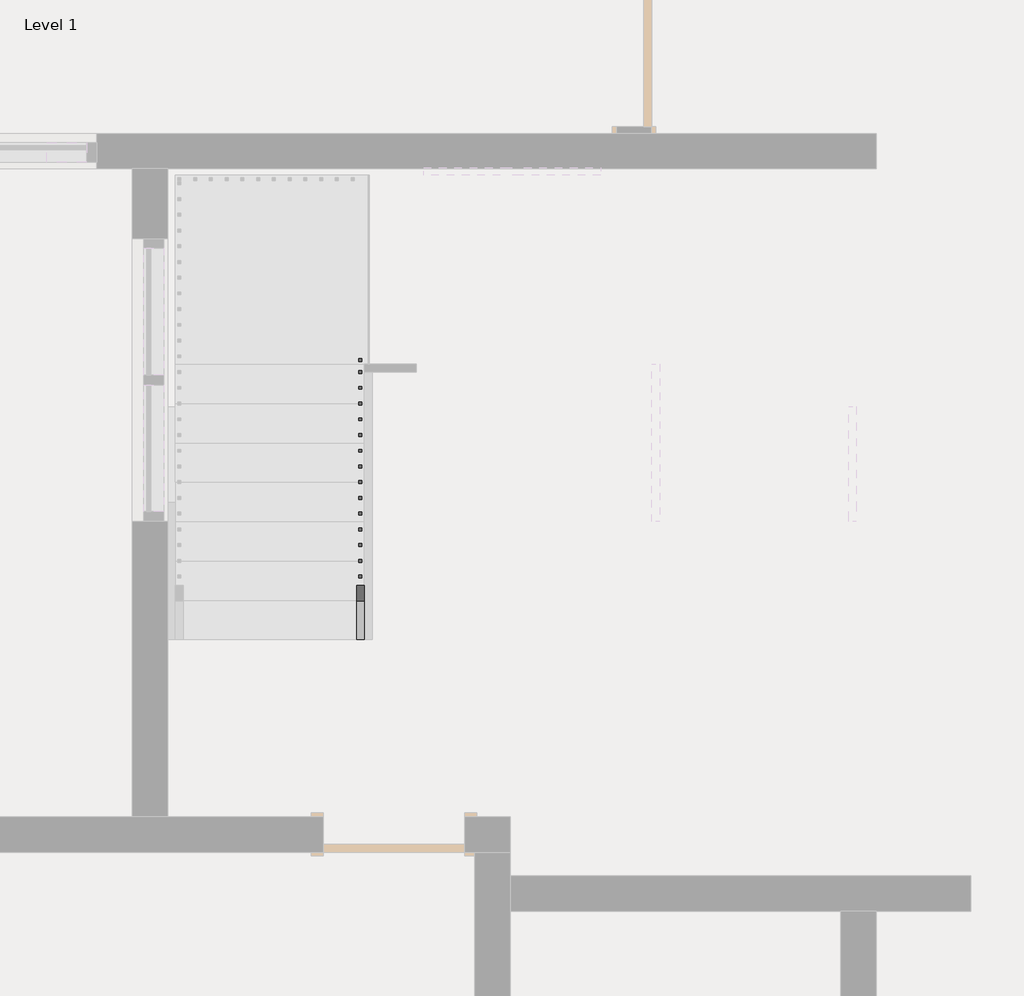
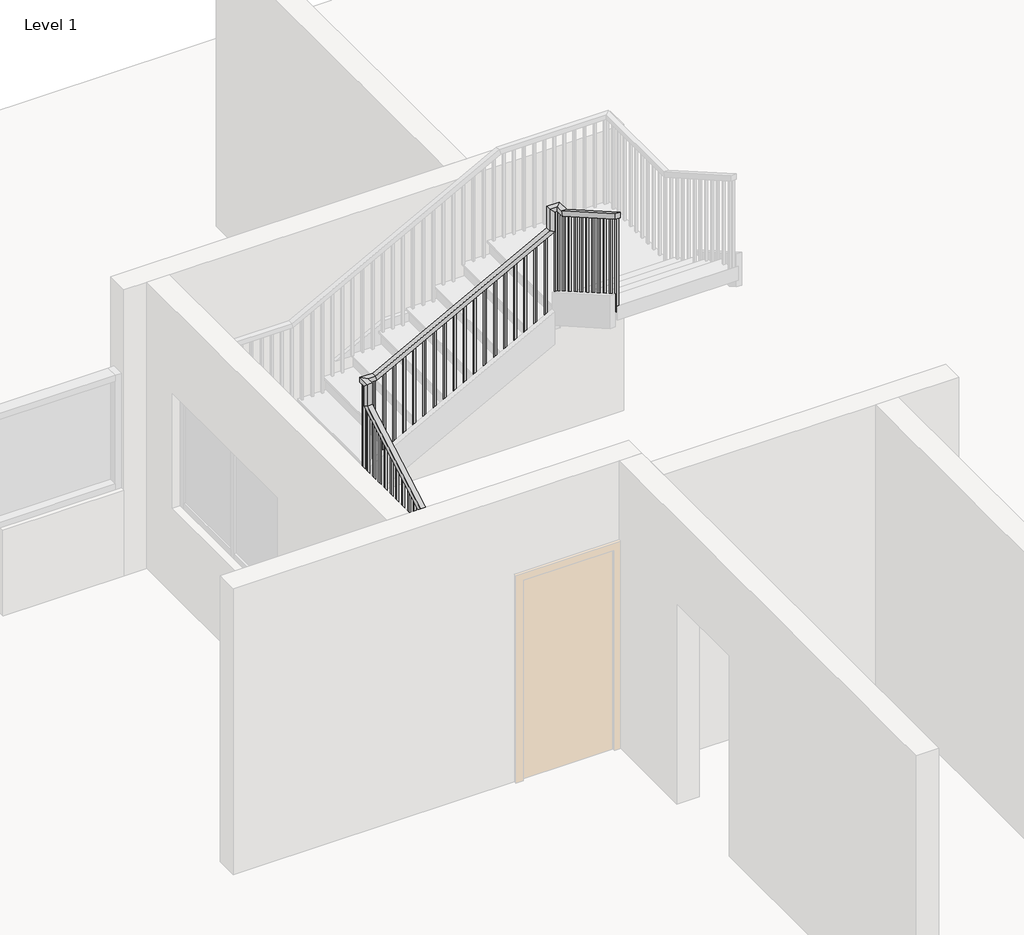
# One storey, part 6 of 9: 1 railing.
"""IFC4 building model written with IfcOpenShell, lengths in millimetres."""

from ifc_helpers import new_model, si_unit, frame, origin, place, context, project, spatial, polyline, outline, extrude, faceted_brep, element, save

model = new_model("IFC4")

# Units and contexts
model_context = context("Model", 3, world=origin())
ifc_project = project(units=[si_unit("LENGTHUNIT", "METRE", prefix="MILLI")], contexts=[model_context])

# Site, building, storey
site = spatial("IfcSite", under=ifc_project)
building = spatial("IfcBuilding", under=site)
storey = spatial("IfcBuildingStorey", under=building, Name="Level 1", Elevation=0.0)

# Railing
placement = place(None, origin())
element("IfcRailing", 1, ObjectType="Handrail - Rectangular", at=placement, inside=storey, context=model_context, shape_type="SolidModel", body=[
    faceted_brep([(-39782.5146233, 12415.3624892, 1059.5428571), (-39782.5146233, 12415.3624892, 1001.0339009), (-39731.7146233, 12415.3624892, 1001.0339009), (-39731.7146233, 12415.3624892, 1059.5428571), (-39782.5146233, 14117.1624892, 2032.0), (-39782.5146233, 14167.9624892, 2002.5196152), (-39731.7146233, 14167.9624892, 2002.5196152), (-39731.7146233, 14117.1624892, 2032.0), (-39782.5146233, 14117.1624892, 2261.3257143), (-39782.5146233, 14167.9624892, 2210.5257143), (-39731.7146233, 14167.9624892, 2210.5257143), (-39731.7146233, 14117.1624892, 2261.3257143), (-39782.5146233, 14244.1624892, 2261.3257143), (-39782.5146233, 14244.1624892, 2210.5257143), (-39731.7146233, 14193.3624892, 2210.5257143), (-39731.7146233, 14193.3624892, 2261.3257143), (-39655.5146233, 14244.1624892, 2261.3257143), (-39642.8146233, 14244.1624892, 2210.5257143), (-39642.8146233, 14193.3624892, 2210.5257143), (-39655.5146233, 14193.3624892, 2261.3257143), (-37902.9146233, 14244.1624892, 3196.0457143), (-37852.1146233, 14244.1624892, 3165.5657143), (-37852.1146233, 14193.3624892, 3165.5657143), (-37902.9146233, 14193.3624892, 3196.0457143), (-37902.9146233, 14244.1624892, 3425.3714286), (-37852.1146233, 14244.1624892, 3374.5714286), (-37852.1146233, 14193.3624892, 3374.5714286), (-37902.9146233, 14193.3624892, 3425.3714286), (-37775.9146233, 14244.1624892, 3425.3714286), (-37775.9146233, 14244.1624892, 3374.5714286), (-37826.7146233, 14193.3624892, 3374.5714286), (-37826.7146233, 14193.3624892, 3425.3714286), (-37775.9146233, 14117.1624892, 3425.3714286), (-37775.9146233, 14103.6718158, 3374.5714286), (-37826.7146233, 14103.6718158, 3374.5714286), (-37826.7146233, 14117.1624892, 3425.3714286), (-37775.9146233, 13177.3624892, 3962.4), (-37826.7146233, 13177.3624892, 3962.4), (-37826.7146233, 13177.3624892, 3903.8910438), (-37775.9146233, 13177.3624892, 3903.8910438)], [[[0, 1, 2, 3]], [[1, 0, 4, 5]], [[2, 1, 5, 6]], [[3, 2, 6, 7]], [[0, 3, 7, 4]], [[5, 4, 8, 9]], [[6, 5, 9, 10]], [[7, 6, 10, 11]], [[4, 7, 11, 8]], [[9, 8, 12, 13]], [[10, 9, 13, 14]], [[11, 10, 14, 15]], [[8, 11, 15, 12]], [[13, 12, 16, 17]], [[14, 13, 17, 18]], [[15, 14, 18, 19]], [[12, 15, 19, 16]], [[17, 16, 20, 21]], [[18, 17, 21, 22]], [[19, 18, 22, 23]], [[16, 19, 23, 20]], [[21, 20, 24, 25]], [[22, 21, 25, 26]], [[23, 22, 26, 27]], [[20, 23, 27, 24]], [[25, 24, 28, 29]], [[26, 25, 29, 30]], [[27, 26, 30, 31]], [[24, 27, 31, 28]], [[29, 28, 32, 33]], [[30, 29, 33, 34]], [[31, 30, 34, 35]], [[28, 31, 35, 32]], [[36, 37, 38, 39]], [[33, 32, 36, 39]], [[34, 33, 39, 38]], [[35, 34, 38, 37]], [[32, 35, 37, 36]]]),
    extrude(outline(polyline([(13193.2374892, 3894.8196152), (13212.2874892, 3883.9339009), (13212.2874892, 2902.8571429), (13193.2374892, 2902.8571429), (13193.2374892, 3894.8196152)])), frame((-37810.8396233, 0.0, 0.0), z_axis=(1.0, 0.0, 0.0), x_axis=(0.0, 1.0, 0.0)), (0.0, 0.0, 1.0), 19.05),
    extrude(outline(polyline([(13294.8374892, 3836.7624723), (13313.8874892, 3825.8767581), (13313.8874892, 2902.8571429), (13294.8374892, 2902.8571429), (13294.8374892, 3836.7624723)])), frame((-37810.8396233, 0.0, 0.0), z_axis=(1.0, 0.0, 0.0), x_axis=(0.0, 1.0, 0.0)), (0.0, 0.0, 1.0), 19.05),
    extrude(outline(polyline([(13396.4374892, 3778.7053295), (13415.4874892, 3767.8196152), (13415.4874892, 2902.8571429), (13396.4374892, 2902.8571429), (13396.4374892, 3778.7053295)])), frame((-37810.8396233, 0.0, 0.0), z_axis=(1.0, 0.0, 0.0), x_axis=(0.0, 1.0, 0.0)), (0.0, 0.0, 1.0), 19.05),
    extrude(outline(polyline([(13498.0374892, 3720.6481866), (13517.0874892, 3709.7624723), (13517.0874892, 2757.7142857), (13498.0374892, 2757.7142857), (13498.0374892, 3720.6481866)])), frame((-37810.8396233, 0.0, 0.0), z_axis=(1.0, 0.0, 0.0), x_axis=(0.0, 1.0, 0.0)), (0.0, 0.0, 1.0), 19.05),
    extrude(outline(polyline([(13599.6374892, 3662.5910438), (13618.6874892, 3651.7053295), (13618.6874892, 2757.7142857), (13599.6374892, 2757.7142857), (13599.6374892, 3662.5910438)])), frame((-37810.8396233, 0.0, 0.0), z_axis=(1.0, 0.0, 0.0), x_axis=(0.0, 1.0, 0.0)), (0.0, 0.0, 1.0), 19.05),
    extrude(outline(polyline([(13701.2374892, 3604.5339009), (13720.2874892, 3593.6481866), (13720.2874892, 2612.5714286), (13701.2374892, 2612.5714286), (13701.2374892, 3604.5339009)])), frame((-37810.8396233, 0.0, 0.0), z_axis=(1.0, 0.0, 0.0), x_axis=(0.0, 1.0, 0.0)), (0.0, 0.0, 1.0), 19.05),
    extrude(outline(polyline([(13802.8374892, 3546.4767581), (13821.8874892, 3535.5910438), (13821.8874892, 2612.5714286), (13802.8374892, 2612.5714286), (13802.8374892, 3546.4767581)])), frame((-37810.8396233, 0.0, 0.0), z_axis=(1.0, 0.0, 0.0), x_axis=(0.0, 1.0, 0.0)), (0.0, 0.0, 1.0), 19.05),
    extrude(outline(polyline([(13904.4374892, 3488.4196152), (13923.4874892, 3477.5339009), (13923.4874892, 2612.5714286), (13904.4374892, 2612.5714286), (13904.4374892, 3488.4196152)])), frame((-37810.8396233, 0.0, 0.0), z_axis=(1.0, 0.0, 0.0), x_axis=(0.0, 1.0, 0.0)), (0.0, 0.0, 1.0), 19.05),
    extrude(outline(polyline([(14006.0374892, 3430.3624723), (14025.0874892, 3419.4767581), (14025.0874892, 2467.4285714), (14006.0374892, 2467.4285714), (14006.0374892, 3430.3624723)])), frame((-37810.8396233, 0.0, 0.0), z_axis=(1.0, 0.0, 0.0), x_axis=(0.0, 1.0, 0.0)), (0.0, 0.0, 1.0), 19.05),
    extrude(outline(polyline([(14107.6374892, 3372.3053295), (14126.6874892, 3361.4196152), (14126.6874892, 2467.4285714), (14107.6374892, 2467.4285714), (14107.6374892, 3372.3053295)])), frame((-37810.8396233, 0.0, 0.0), z_axis=(1.0, 0.0, 0.0), x_axis=(0.0, 1.0, 0.0)), (0.0, 0.0, 1.0), 19.05),
    extrude(outline(polyline([(-37836.2396233, 14209.2374892), (-37836.2396233, 14228.2874892), (-37817.1896233, 14228.2874892), (-37817.1896233, 14209.2374892), (-37836.2396233, 14209.2374892)])), frame((0.0, 0.0, 2322.2857143), z_axis=(0.0, 0.0, 1.0), x_axis=(1.0, 0.0, 0.0)), (0.0, 0.0, 1.0), 1052.2857143),
    extrude(outline(polyline([(3130.0057143, -37918.7896233), (3119.8457143, -37937.8396233), (2177.1428571, -37937.8396233), (2177.1428571, -37918.7896233), (3130.0057143, -37918.7896233)])), frame((0.0, 14209.2374892, 0.0), z_axis=(0.0, 1.0, 0.0), x_axis=(0.0, 0.0, 1.0)), (0.0, 0.0, 1.0), 19.05),
    extrude(outline(polyline([(3075.8190476, -38020.3896233), (3065.6590476, -38039.4396233), (2177.1428571, -38039.4396233), (2177.1428571, -38020.3896233), (3075.8190476, -38020.3896233)])), frame((0.0, 14209.2374892, 0.0), z_axis=(0.0, 1.0, 0.0), x_axis=(0.0, 0.0, 1.0)), (0.0, 0.0, 1.0), 19.05),
    extrude(outline(polyline([(3021.632381, -38121.9896233), (3011.472381, -38141.0396233), (2032.0, -38141.0396233), (2032.0, -38121.9896233), (3021.632381, -38121.9896233)])), frame((0.0, 14209.2374892, 0.0), z_axis=(0.0, 1.0, 0.0), x_axis=(0.0, 0.0, 1.0)), (0.0, 0.0, 1.0), 19.05),
    extrude(outline(polyline([(2967.4457143, -38223.5896233), (2957.2857143, -38242.6396233), (2032.0, -38242.6396233), (2032.0, -38223.5896233), (2967.4457143, -38223.5896233)])), frame((0.0, 14209.2374892, 0.0), z_axis=(0.0, 1.0, 0.0), x_axis=(0.0, 0.0, 1.0)), (0.0, 0.0, 1.0), 19.05),
    extrude(outline(polyline([(2913.2590476, -38325.1896233), (2903.0990476, -38344.2396233), (2032.0, -38344.2396233), (2032.0, -38325.1896233), (2913.2590476, -38325.1896233)])), frame((0.0, 14209.2374892, 0.0), z_axis=(0.0, 1.0, 0.0), x_axis=(0.0, 0.0, 1.0)), (0.0, 0.0, 1.0), 19.05),
    extrude(outline(polyline([(2859.072381, -38426.7896233), (2848.912381, -38445.8396233), (1886.8571429, -38445.8396233), (1886.8571429, -38426.7896233), (2859.072381, -38426.7896233)])), frame((0.0, 14209.2374892, 0.0), z_axis=(0.0, 1.0, 0.0), x_axis=(0.0, 0.0, 1.0)), (0.0, 0.0, 1.0), 19.05),
    extrude(outline(polyline([(2804.8857143, -38528.3896233), (2794.7257143, -38547.4396233), (1886.8571429, -38547.4396233), (1886.8571429, -38528.3896233), (2804.8857143, -38528.3896233)])), frame((0.0, 14209.2374892, 0.0), z_axis=(0.0, 1.0, 0.0), x_axis=(0.0, 0.0, 1.0)), (0.0, 0.0, 1.0), 19.05),
    extrude(outline(polyline([(2750.6990476, -38629.9896233), (2740.5390476, -38649.0396233), (1886.8571429, -38649.0396233), (1886.8571429, -38629.9896233), (2750.6990476, -38629.9896233)])), frame((0.0, 14209.2374892, 0.0), z_axis=(0.0, 1.0, 0.0), x_axis=(0.0, 0.0, 1.0)), (0.0, 0.0, 1.0), 19.05),
    extrude(outline(polyline([(2696.512381, -38731.5896233), (2686.352381, -38750.6396233), (1741.7142857, -38750.6396233), (1741.7142857, -38731.5896233), (2696.512381, -38731.5896233)])), frame((0.0, 14209.2374892, 0.0), z_axis=(0.0, 1.0, 0.0), x_axis=(0.0, 0.0, 1.0)), (0.0, 0.0, 1.0), 19.05),
    extrude(outline(polyline([(2642.3257143, -38833.1896233), (2632.1657143, -38852.2396233), (1741.7142857, -38852.2396233), (1741.7142857, -38833.1896233), (2642.3257143, -38833.1896233)])), frame((0.0, 14209.2374892, 0.0), z_axis=(0.0, 1.0, 0.0), x_axis=(0.0, 0.0, 1.0)), (0.0, 0.0, 1.0), 19.05),
    extrude(outline(polyline([(2588.1390476, -38934.7896233), (2577.9790476, -38953.8396233), (1596.5714286, -38953.8396233), (1596.5714286, -38934.7896233), (2588.1390476, -38934.7896233)])), frame((0.0, 14209.2374892, 0.0), z_axis=(0.0, 1.0, 0.0), x_axis=(0.0, 0.0, 1.0)), (0.0, 0.0, 1.0), 19.05),
    extrude(outline(polyline([(2533.952381, -39036.3896233), (2523.792381, -39055.4396233), (1596.5714286, -39055.4396233), (1596.5714286, -39036.3896233), (2533.952381, -39036.3896233)])), frame((0.0, 14209.2374892, 0.0), z_axis=(0.0, 1.0, 0.0), x_axis=(0.0, 0.0, 1.0)), (0.0, 0.0, 1.0), 19.05),
    extrude(outline(polyline([(2479.7657143, -39137.9896233), (2469.6057143, -39157.0396233), (1596.5714286, -39157.0396233), (1596.5714286, -39137.9896233), (2479.7657143, -39137.9896233)])), frame((0.0, 14209.2374892, 0.0), z_axis=(0.0, 1.0, 0.0), x_axis=(0.0, 0.0, 1.0)), (0.0, 0.0, 1.0), 19.05),
    extrude(outline(polyline([(2425.5790476, -39239.5896233), (2415.4190476, -39258.6396233), (1451.4285714, -39258.6396233), (1451.4285714, -39239.5896233), (2425.5790476, -39239.5896233)])), frame((0.0, 14209.2374892, 0.0), z_axis=(0.0, 1.0, 0.0), x_axis=(0.0, 0.0, 1.0)), (0.0, 0.0, 1.0), 19.05),
    extrude(outline(polyline([(2371.392381, -39341.1896233), (2361.232381, -39360.2396233), (1451.4285714, -39360.2396233), (1451.4285714, -39341.1896233), (2371.392381, -39341.1896233)])), frame((0.0, 14209.2374892, 0.0), z_axis=(0.0, 1.0, 0.0), x_axis=(0.0, 0.0, 1.0)), (0.0, 0.0, 1.0), 19.05),
    extrude(outline(polyline([(2317.2057143, -39442.7896233), (2307.0457143, -39461.8396233), (1451.4285714, -39461.8396233), (1451.4285714, -39442.7896233), (2317.2057143, -39442.7896233)])), frame((0.0, 14209.2374892, 0.0), z_axis=(0.0, 1.0, 0.0), x_axis=(0.0, 0.0, 1.0)), (0.0, 0.0, 1.0), 19.05),
    extrude(outline(polyline([(2263.0190476, -39544.3896233), (2252.8590476, -39563.4396233), (1306.2857143, -39563.4396233), (1306.2857143, -39544.3896233), (2263.0190476, -39544.3896233)])), frame((0.0, 14209.2374892, 0.0), z_axis=(0.0, 1.0, 0.0), x_axis=(0.0, 0.0, 1.0)), (0.0, 0.0, 1.0), 19.05),
    extrude(outline(polyline([(2208.832381, -39645.9896233), (2198.672381, -39665.0396233), (1306.2857143, -39665.0396233), (1306.2857143, -39645.9896233), (2208.832381, -39645.9896233)])), frame((0.0, 14209.2374892, 0.0), z_axis=(0.0, 1.0, 0.0), x_axis=(0.0, 0.0, 1.0)), (0.0, 0.0, 1.0), 19.05),
    extrude(outline(polyline([(-39747.5896233, 14133.0374892), (-39766.6396233, 14133.0374892), (-39766.6396233, 14152.0874892), (-39747.5896233, 14152.0874892), (-39747.5896233, 14133.0374892)])), frame((0.0, 0.0, 1016.0), z_axis=(0.0, 0.0, 1.0), x_axis=(1.0, 0.0, 0.0)), (0.0, 0.0, 1.0), 1194.5257143),
    extrude(outline(polyline([(14031.4374892, 1924.5053295), (14050.4874892, 1935.3910438), (14050.4874892, 1016.0), (14031.4374892, 1016.0), (14031.4374892, 1924.5053295)])), frame((-39766.6396233, 0.0, 0.0), z_axis=(1.0, 0.0, 0.0), x_axis=(0.0, 1.0, 0.0)), (0.0, 0.0, 1.0), 19.05),
    extrude(outline(polyline([(13929.8374892, 1866.4481866), (13948.8874892, 1877.3339009), (13948.8874892, 1016.0), (13929.8374892, 1016.0), (13929.8374892, 1866.4481866)])), frame((-39766.6396233, 0.0, 0.0), z_axis=(1.0, 0.0, 0.0), x_axis=(0.0, 1.0, 0.0)), (0.0, 0.0, 1.0), 19.05),
    extrude(outline(polyline([(13828.2374892, 1808.3910438), (13847.2874892, 1819.2767581), (13847.2874892, 870.8571429), (13828.2374892, 870.8571429), (13828.2374892, 1808.3910438)])), frame((-39766.6396233, 0.0, 0.0), z_axis=(1.0, 0.0, 0.0), x_axis=(0.0, 1.0, 0.0)), (0.0, 0.0, 1.0), 19.05),
    extrude(outline(polyline([(13726.6374892, 1750.3339009), (13745.6874892, 1761.2196152), (13745.6874892, 870.8571429), (13726.6374892, 870.8571429), (13726.6374892, 1750.3339009)])), frame((-39766.6396233, 0.0, 0.0), z_axis=(1.0, 0.0, 0.0), x_axis=(0.0, 1.0, 0.0)), (0.0, 0.0, 1.0), 19.05),
    extrude(outline(polyline([(13625.0374892, 1692.2767581), (13644.0874892, 1703.1624723), (13644.0874892, 725.7142857), (13625.0374892, 725.7142857), (13625.0374892, 1692.2767581)])), frame((-39766.6396233, 0.0, 0.0), z_axis=(1.0, 0.0, 0.0), x_axis=(0.0, 1.0, 0.0)), (0.0, 0.0, 1.0), 19.05),
    extrude(outline(polyline([(13523.4374892, 1634.2196152), (13542.4874892, 1645.1053295), (13542.4874892, 725.7142857), (13523.4374892, 725.7142857), (13523.4374892, 1634.2196152)])), frame((-39766.6396233, 0.0, 0.0), z_axis=(1.0, 0.0, 0.0), x_axis=(0.0, 1.0, 0.0)), (0.0, 0.0, 1.0), 19.05),
    extrude(outline(polyline([(13421.8374892, 1576.1624723), (13440.8874892, 1587.0481866), (13440.8874892, 725.7142857), (13421.8374892, 725.7142857), (13421.8374892, 1576.1624723)])), frame((-39766.6396233, 0.0, 0.0), z_axis=(1.0, 0.0, 0.0), x_axis=(0.0, 1.0, 0.0)), (0.0, 0.0, 1.0), 19.05),
    extrude(outline(polyline([(13320.2374892, 1518.1053295), (13339.2874892, 1528.9910438), (13339.2874892, 580.5714286), (13320.2374892, 580.5714286), (13320.2374892, 1518.1053295)])), frame((-39766.6396233, 0.0, 0.0), z_axis=(1.0, 0.0, 0.0), x_axis=(0.0, 1.0, 0.0)), (0.0, 0.0, 1.0), 19.05),
    extrude(outline(polyline([(13218.6374892, 1460.0481866), (13237.6874892, 1470.9339009), (13237.6874892, 580.5714286), (13218.6374892, 580.5714286), (13218.6374892, 1460.0481866)])), frame((-39766.6396233, 0.0, 0.0), z_axis=(1.0, 0.0, 0.0), x_axis=(0.0, 1.0, 0.0)), (0.0, 0.0, 1.0), 19.05),
    extrude(outline(polyline([(13117.0374892, 1401.9910438), (13136.0874892, 1412.8767581), (13136.0874892, 435.4285714), (13117.0374892, 435.4285714), (13117.0374892, 1401.9910438)])), frame((-39766.6396233, 0.0, 0.0), z_axis=(1.0, 0.0, 0.0), x_axis=(0.0, 1.0, 0.0)), (0.0, 0.0, 1.0), 19.05),
    extrude(outline(polyline([(13015.4374892, 1343.9339009), (13034.4874892, 1354.8196152), (13034.4874892, 435.4285714), (13015.4374892, 435.4285714), (13015.4374892, 1343.9339009)])), frame((-39766.6396233, 0.0, 0.0), z_axis=(1.0, 0.0, 0.0), x_axis=(0.0, 1.0, 0.0)), (0.0, 0.0, 1.0), 19.05),
    extrude(outline(polyline([(12913.8374892, 1285.8767581), (12932.8874892, 1296.7624723), (12932.8874892, 435.4285714), (12913.8374892, 435.4285714), (12913.8374892, 1285.8767581)])), frame((-39766.6396233, 0.0, 0.0), z_axis=(1.0, 0.0, 0.0), x_axis=(0.0, 1.0, 0.0)), (0.0, 0.0, 1.0), 19.05),
    extrude(outline(polyline([(12812.2374892, 1227.8196152), (12831.2874892, 1238.7053295), (12831.2874892, 290.2857143), (12812.2374892, 290.2857143), (12812.2374892, 1227.8196152)])), frame((-39766.6396233, 0.0, 0.0), z_axis=(1.0, 0.0, 0.0), x_axis=(0.0, 1.0, 0.0)), (0.0, 0.0, 1.0), 19.05),
    extrude(outline(polyline([(12710.6374892, 1169.7624723), (12729.6874892, 1180.6481866), (12729.6874892, 290.2857143), (12710.6374892, 290.2857143), (12710.6374892, 1169.7624723)])), frame((-39766.6396233, 0.0, 0.0), z_axis=(1.0, 0.0, 0.0), x_axis=(0.0, 1.0, 0.0)), (0.0, 0.0, 1.0), 19.05),
    extrude(outline(polyline([(12609.0374892, 1111.7053295), (12628.0874892, 1122.5910438), (12628.0874892, 145.1428571), (12609.0374892, 145.1428571), (12609.0374892, 1111.7053295)])), frame((-39766.6396233, 0.0, 0.0), z_axis=(1.0, 0.0, 0.0), x_axis=(0.0, 1.0, 0.0)), (0.0, 0.0, 1.0), 19.05),
    extrude(outline(polyline([(12507.4374892, 1053.6481866), (12526.4874892, 1064.5339009), (12526.4874892, 145.1428571), (12507.4374892, 145.1428571), (12507.4374892, 1053.6481866)])), frame((-39766.6396233, 0.0, 0.0), z_axis=(1.0, 0.0, 0.0), x_axis=(0.0, 1.0, 0.0)), (0.0, 0.0, 1.0), 19.05),
    extrude(outline(polyline([(-37810.8396233, 14209.2374892), (-37810.8396233, 14228.2874892), (-37791.7896233, 14228.2874892), (-37791.7896233, 14209.2374892), (-37810.8396233, 14209.2374892)])), frame((0.0, 0.0, 2322.2857143), z_axis=(0.0, 0.0, 1.0), x_axis=(1.0, 0.0, 0.0)), (0.0, 0.0, 1.0), 1052.2857143),
    extrude(outline(polyline([(-39747.5896233, 14209.2374892), (-39766.6396233, 14209.2374892), (-39766.6396233, 14228.2874892), (-39747.5896233, 14228.2874892), (-39747.5896233, 14209.2374892)])), frame((0.0, 0.0, 1161.1428571), z_axis=(0.0, 0.0, 1.0), x_axis=(1.0, 0.0, 0.0)), (0.0, 0.0, 1.0), 1049.3828571),
    extrude(outline(polyline([(13177.3624892, 3903.8910438), (13196.4124892, 3893.0053295), (13196.4124892, 2902.8571429), (13177.3624892, 2902.8571429), (13177.3624892, 3903.8910438)])), frame((-37810.8396233, 0.0, 0.0), z_axis=(1.0, 0.0, 0.0), x_axis=(0.0, 1.0, 0.0)), (0.0, 0.0, 1.0), 19.05),
    extrude(outline(polyline([(12415.3624892, 1001.0339009), (12434.4124892, 1011.9196152), (12434.4124892, 145.1428571), (12415.3624892, 145.1428571), (12415.3624892, 1001.0339009)])), frame((-39766.6396233, 0.0, 0.0), z_axis=(1.0, 0.0, 0.0), x_axis=(0.0, 1.0, 0.0)), (0.0, 0.0, 1.0), 19.05),
])

save(model, "model.ifc")

# Revit data of these elements
# Type "Handrail - Rectangular"
#   Assembly Code = "C2010400"
#   built-in parameter 1008612 = 0.0416667 (stored number, unit not read)
#   built-in parameter 1008611 = 0.0416667 (stored number, unit not read)
#   built-in parameter 1008609 = 0.333333 (stored number, unit not read)
#   built-in parameter 1008604 = 0.166667 (stored number, unit not read)
#   built-in parameter 1008603 = 0.166667 (stored number, unit not read)
#   Railing Height = 3' - 0"
#   built-in parameter 1008630 = 2
#   built-in parameter 1008610 = 2
#   built-in parameter 1008618 = Baluster - Square : 3/4"
# Element 1 (IfcRailing, "Handrail - Rectangular")
#   Phase Created = New Construction
